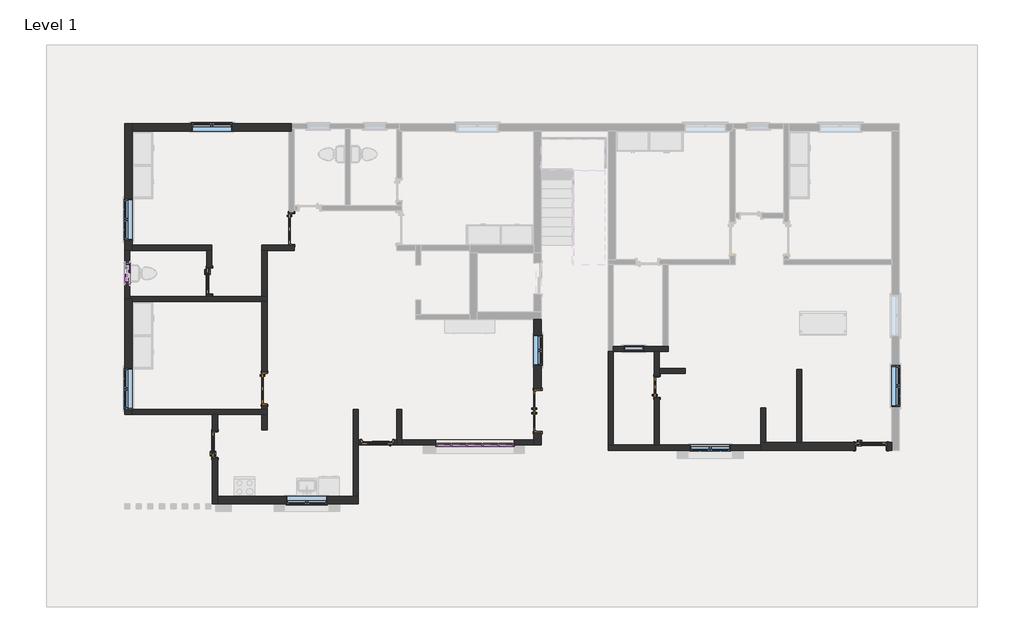
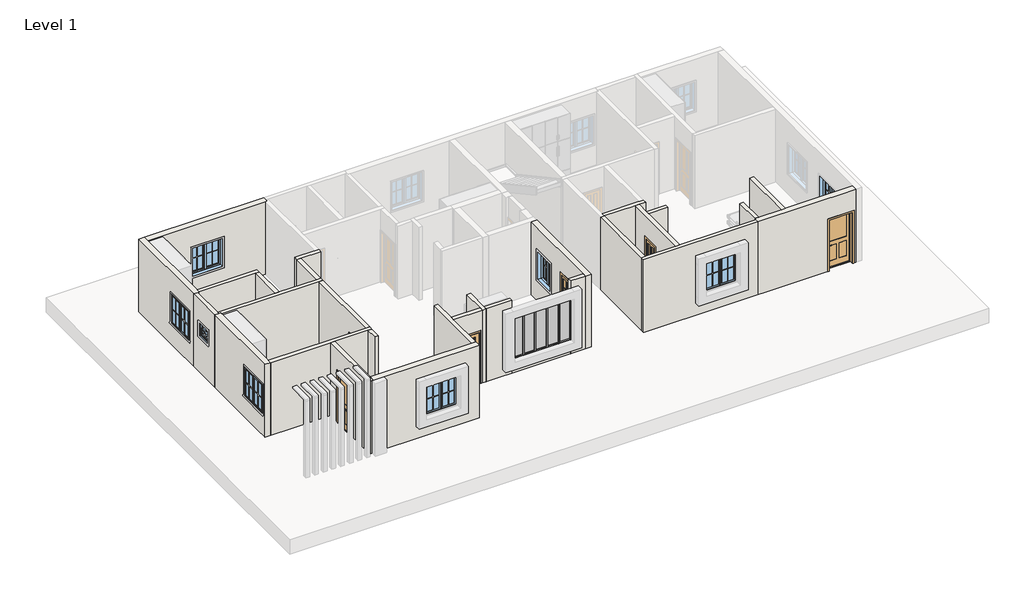
# One storey, part 1 of 3: 29 walls, 16 members, 9 windows, 8 doors, 5 plates.
"""IFC4 building model written with IfcOpenShell, lengths in millimetres."""

from ifc_helpers import new_model, si_unit, frame, origin, origin_with_axes, place, context, project, spatial, polyline, outline, extrude, faceted_brep, transform, mapped, element, save
from components import door_c9530512, door_0459eae1, door_3_x_7_64fb43ed, door_exterior_single_two_lite_3_x_7_37050820, door_interior_double_full_glass_wood_md_4_x_7_6b6f14de, door_interior_single_4_panel_wood_2_x_7_099afc9e, door_interior_single_4_panel_wood_bed_door_3_x_7_5a83478c, member_f5dffbef, member_20da7b42, member_5c57b440, member_8587bb6c, member_65702978, member_b71d7755, system_panel_glazed_d030299f, system_panel_glazed_4b6a6dc2, system_panel_glazed_d31e9b5d, system_panel_glazed_e2ad0beb, window_casement_double_3_x_4_2abbe05e, window_casement_double_4_x_4_9200f5ac, window_casement_double_4_x_4_83c2abfa, window_double_hung_2_x_2_0206a36d

model = new_model("IFC4")

# Units and contexts
model_context = context("Model", 3, world=origin())
ifc_project = project(units=[si_unit("LENGTHUNIT", "METRE", prefix="MILLI")], contexts=[model_context])

# Site, building, storey
site = spatial("IfcSite", under=ifc_project)
building = spatial("IfcBuilding", under=site)
storey = spatial("IfcBuildingStorey", under=building, Name="Level 1", Elevation=0.0)

# Doors
placement = place(None, origin())
door_shape = door_c9530512(model_context)
element("IfcDoor", 1, ObjectType="2'6\" X 7'", at=placement, inside=storey, context=model_context, shape_type="MappedRepresentation", body=[
    mapped(door_shape, transform((-9422.3392415, -3706.312639, 0.0), x_axis=(0.0, -1.0, 0.0), y_axis=(1.0, 0.0, 0.0), z_axis=(0.0, 0.0, 1.0))),
])
door_2_shape = door_0459eae1(model_context)
element("IfcDoor", 2, ObjectType="2'6\" X 7'", at=placement, inside=storey, context=model_context, shape_type="MappedRepresentation", body=[
    mapped(door_2_shape, transform((-9588.7286806, 1157.6726898, 0.0), x_axis=(0.0, 1.0, 0.0), y_axis=(-1.0, 0.0, 0.0), z_axis=(0.0, 0.0, 1.0))),
])
door_3_x_7_shape = door_3_x_7_64fb43ed(model_context)
element("IfcDoor", 3, ObjectType="3' X 7'", at=placement, inside=storey, context=model_context, shape_type="MappedRepresentation", body=[
    mapped(door_3_x_7_shape, transform((10074.0463194, -3754.0523102, 0.0), x_axis=(-1.0, 0.0, 0.0), y_axis=(0.0, -1.0, 0.0), z_axis=(0.0, 0.0, 1.0))),
])
door_exterior_single_two_lite_3_x_7_shape = door_exterior_single_two_lite_3_x_7_37050820(model_context)
element("IfcDoor", 4, ObjectType="Door-Exterior-Single-Two_Lite : 3' x 7'", at=placement, inside=storey, context=model_context, shape_type="MappedRepresentation", body=[
    mapped(door_exterior_single_two_lite_3_x_7_shape, transform((-4594.4536806, -3636.5773102, 0.0), x_axis=(-1.0, 0.0, 0.0), y_axis=(0.0, -1.0, 0.0), z_axis=(0.0, 0.0, 1.0))),
])
door_interior_double_full_glass_wood_md_4_x_7_shape = door_interior_double_full_glass_wood_md_4_x_7_6b6f14de(model_context)
element("IfcDoor", 5, ObjectType="Door-Interior-Double-Full Glass-Wood : MD 4' X 7'", at=placement, inside=storey, context=model_context, shape_type="MappedRepresentation", body=[
    mapped(door_interior_double_full_glass_wood_md_4_x_7_shape, transform((164.8713194, -2703.1273102, 0.0), x_axis=(0.0, 1.0, 0.0), y_axis=(-1.0, 0.0, 0.0), z_axis=(0.0, 0.0, 1.0))),
])
door_interior_single_4_panel_wood_2_x_7_shape = door_interior_single_4_panel_wood_2_x_7_099afc9e(model_context)
element("IfcDoor", 6, ObjectType="Door-Interior-Single-4_Panel-Wood : 2' X 7'", at=placement, inside=storey, context=model_context, shape_type="MappedRepresentation", body=[
    mapped(door_interior_single_4_panel_wood_2_x_7_shape, transform((3708.1713194, -1991.9273102, 0.0), x_axis=(0.0, 1.0, 0.0), y_axis=(-1.0, 0.0, 0.0), z_axis=(0.0, 0.0, 1.0))),
])
door_interior_single_4_panel_wood_bed_door_3_x_7_shape = door_interior_single_4_panel_wood_bed_door_3_x_7_5a83478c(model_context)
element("IfcDoor", 7, ObjectType="Door-Interior-Single-4_Panel-Wood : BED DOOR 3' X 7'", at=placement, inside=storey, context=model_context, shape_type="MappedRepresentation", body=[
    mapped(door_interior_single_4_panel_wood_bed_door_3_x_7_shape, transform((-7150.3286806, 2700.7226898, 0.0), x_axis=(0.0, -1.0, 0.0), y_axis=(1.0, 0.0, 0.0), z_axis=(0.0, 0.0, 1.0))),
])
element("IfcDoor", 8, ObjectType="Door-Interior-Single-4_Panel-Wood : BED DOOR 3' X 7'", at=placement, inside=storey, context=model_context, shape_type="MappedRepresentation", body=[
    mapped(door_interior_single_4_panel_wood_bed_door_3_x_7_shape, transform((-7950.4286806, -2042.7273102, 0.0), x_axis=(0.0, -1.0, 0.0), y_axis=(1.0, 0.0, 0.0), z_axis=(0.0, 0.0, 1.0))),
])

# Members
member_shape = member_f5dffbef(model_context)
element("IfcMember", 9, ObjectType="Rectangular Mullion : 1.5\" x 2.5\" rectangular", at=placement, inside=storey, context=model_context, shape_type="MappedRepresentation", body=[
    mapped(member_shape, transform((-568.5536806, -3719.1273102, 2438.4), x_axis=(0.0, 0.0, 1.0), y_axis=(0.0, -1.0, 0.0), z_axis=(1.0, 0.0, 0.0))),
])
member_2_shape = member_20da7b42(model_context)
element("IfcMember", 10, ObjectType="Rectangular Mullion : 1.5\" x 2.5\" rectangular", at=placement, inside=storey, context=model_context, shape_type="MappedRepresentation", body=[
    mapped(member_2_shape, transform((-2816.4536806, -3719.1273102, 609.6), x_axis=(0.0, 0.0, -1.0), y_axis=(0.0, -1.0, 0.0), z_axis=(-1.0, 0.0, 0.0))),
])
member_3_shape = member_5c57b440(model_context)
element("IfcMember", 11, ObjectType="Rectangular Mullion : 1.5\" x 2.5\" rectangular", at=placement, inside=storey, context=model_context, shape_type="MappedRepresentation", body=[
    mapped(member_3_shape, transform((-2397.3536806, -3719.1273102, 609.6), x_axis=(1.0, 0.0, 0.0), y_axis=(0.0, -1.0, 0.0), z_axis=(0.0, 0.0, -1.0))),
])
element("IfcMember", 12, ObjectType="Rectangular Mullion : 1.5\" x 2.5\" rectangular", at=placement, inside=storey, context=model_context, shape_type="MappedRepresentation", body=[
    mapped(member_3_shape, transform((-1940.1536806, -3719.1273102, 609.6), x_axis=(1.0, 0.0, 0.0), y_axis=(0.0, -1.0, 0.0), z_axis=(0.0, 0.0, -1.0))),
])
element("IfcMember", 13, ObjectType="Rectangular Mullion : 1.5\" x 2.5\" rectangular", at=placement, inside=storey, context=model_context, shape_type="MappedRepresentation", body=[
    mapped(member_3_shape, transform((-1470.2536806, -3719.1273102, 609.6), x_axis=(1.0, 0.0, 0.0), y_axis=(0.0, -1.0, 0.0), z_axis=(0.0, 0.0, -1.0))),
])
element("IfcMember", 14, ObjectType="Rectangular Mullion : 1.5\" x 2.5\" rectangular", at=placement, inside=storey, context=model_context, shape_type="MappedRepresentation", body=[
    mapped(member_3_shape, transform((-1000.3536806, -3719.1273102, 609.6), x_axis=(1.0, 0.0, 0.0), y_axis=(0.0, -1.0, 0.0), z_axis=(0.0, 0.0, -1.0))),
])
member_4_shape = member_8587bb6c(model_context)
element("IfcMember", 15, ObjectType="Rectangular Mullion : 1.5\" x 2.5\" rectangular", at=placement, inside=storey, context=model_context, shape_type="MappedRepresentation", body=[
    mapped(member_4_shape, transform((-2378.3036806, -3719.1273102, 609.6), x_axis=(0.0, 0.0, -1.0), y_axis=(0.0, -1.0, 0.0), z_axis=(-1.0, 0.0, 0.0))),
])
member_5_shape = member_65702978(model_context)
element("IfcMember", 16, ObjectType="Rectangular Mullion : 1.5\" x 2.5\" rectangular", at=placement, inside=storey, context=model_context, shape_type="MappedRepresentation", body=[
    mapped(member_5_shape, transform((-1921.1036806, -3719.1273102, 609.6), x_axis=(0.0, 0.0, -1.0), y_axis=(0.0, -1.0, 0.0), z_axis=(-1.0, 0.0, 0.0))),
])
element("IfcMember", 17, ObjectType="Rectangular Mullion : 1.5\" x 2.5\" rectangular", at=placement, inside=storey, context=model_context, shape_type="MappedRepresentation", body=[
    mapped(member_5_shape, transform((-1451.2036806, -3719.1273102, 609.6), x_axis=(0.0, 0.0, -1.0), y_axis=(0.0, -1.0, 0.0), z_axis=(-1.0, 0.0, 0.0))),
])
element("IfcMember", 18, ObjectType="Rectangular Mullion : 1.5\" x 2.5\" rectangular", at=placement, inside=storey, context=model_context, shape_type="MappedRepresentation", body=[
    mapped(member_shape, transform((-981.3036806, -3719.1273102, 609.6), x_axis=(0.0, 0.0, -1.0), y_axis=(0.0, -1.0, 0.0), z_axis=(-1.0, 0.0, 0.0))),
])
element("IfcMember", 19, ObjectType="Rectangular Mullion : 1.5\" x 2.5\" rectangular", at=placement, inside=storey, context=model_context, shape_type="MappedRepresentation", body=[
    mapped(member_2_shape, transform((-2416.4036806, -3719.1273102, 2438.4), x_axis=(0.0, 0.0, 1.0), y_axis=(0.0, -1.0, 0.0), z_axis=(1.0, 0.0, 0.0))),
])
element("IfcMember", 20, ObjectType="Rectangular Mullion : 1.5\" x 2.5\" rectangular", at=placement, inside=storey, context=model_context, shape_type="MappedRepresentation", body=[
    mapped(member_4_shape, transform((-1959.2036806, -3719.1273102, 2438.4), x_axis=(0.0, 0.0, 1.0), y_axis=(0.0, -1.0, 0.0), z_axis=(1.0, 0.0, 0.0))),
])
element("IfcMember", 21, ObjectType="Rectangular Mullion : 1.5\" x 2.5\" rectangular", at=placement, inside=storey, context=model_context, shape_type="MappedRepresentation", body=[
    mapped(member_5_shape, transform((-1489.3036806, -3719.1273102, 2438.4), x_axis=(0.0, 0.0, 1.0), y_axis=(0.0, -1.0, 0.0), z_axis=(1.0, 0.0, 0.0))),
])
element("IfcMember", 22, ObjectType="Rectangular Mullion : 1.5\" x 2.5\" rectangular", at=placement, inside=storey, context=model_context, shape_type="MappedRepresentation", body=[
    mapped(member_5_shape, transform((-1019.4036806, -3719.1273102, 2438.4), x_axis=(0.0, 0.0, 1.0), y_axis=(0.0, -1.0, 0.0), z_axis=(1.0, 0.0, 0.0))),
])
member_6_shape = member_b71d7755(model_context)
element("IfcMember", 23, ObjectType="Rectangular Mullion : 1.5\" x 2.5\" rectangular", at=placement, inside=storey, context=model_context, shape_type="MappedRepresentation", body=[
    mapped(member_6_shape, transform((-2854.5536806, -3719.1273102, 2438.4), x_axis=(-1.0, 0.0, 0.0), y_axis=(0.0, -1.0, 0.0), z_axis=(0.0, 0.0, 1.0))),
])
element("IfcMember", 24, ObjectType="Rectangular Mullion : 1.5\" x 2.5\" rectangular", at=placement, inside=storey, context=model_context, shape_type="MappedRepresentation", body=[
    mapped(member_6_shape, transform((-530.4536806, -3719.1273102, 609.6), x_axis=(1.0, 0.0, 0.0), y_axis=(0.0, -1.0, 0.0), z_axis=(0.0, 0.0, -1.0))),
])

# Plates
system_panel_glazed_shape = system_panel_glazed_d030299f(model_context)
element("IfcPlate", 25, ObjectType="System Panel : Glazed", at=placement, inside=storey, context=model_context, shape_type="MappedRepresentation", body=[
    mapped(system_panel_glazed_shape, transform((-2616.4286806, -3719.1273102, 647.7), x_axis=(1.0, 0.0, 0.0), y_axis=(0.0, 1.0, 0.0), z_axis=(0.0, 0.0, 1.0))),
])
system_panel_glazed_2_shape = system_panel_glazed_4b6a6dc2(model_context)
element("IfcPlate", 26, ObjectType="System Panel : Glazed", at=placement, inside=storey, context=model_context, shape_type="MappedRepresentation", body=[
    mapped(system_panel_glazed_2_shape, transform((-2168.7536806, -3719.1273102, 647.7), x_axis=(1.0, 0.0, 0.0), y_axis=(0.0, 1.0, 0.0), z_axis=(0.0, 0.0, 1.0))),
])
system_panel_glazed_3_shape = system_panel_glazed_d31e9b5d(model_context)
element("IfcPlate", 27, ObjectType="System Panel : Glazed", at=placement, inside=storey, context=model_context, shape_type="MappedRepresentation", body=[
    mapped(system_panel_glazed_3_shape, transform((-1705.2036806, -3719.1273102, 647.7), x_axis=(1.0, 0.0, 0.0), y_axis=(0.0, 1.0, 0.0), z_axis=(0.0, 0.0, 1.0))),
])
element("IfcPlate", 28, ObjectType="System Panel : Glazed", at=placement, inside=storey, context=model_context, shape_type="MappedRepresentation", body=[
    mapped(system_panel_glazed_3_shape, transform((-1235.3036806, -3719.1273102, 647.7), x_axis=(1.0, 0.0, 0.0), y_axis=(0.0, 1.0, 0.0), z_axis=(0.0, 0.0, 1.0))),
])
system_panel_glazed_4_shape = system_panel_glazed_e2ad0beb(model_context)
element("IfcPlate", 29, ObjectType="System Panel : Glazed", at=placement, inside=storey, context=model_context, shape_type="MappedRepresentation", body=[
    mapped(system_panel_glazed_4_shape, transform((-774.9286806, -3719.1273102, 647.7), x_axis=(1.0, 0.0, 0.0), y_axis=(0.0, 1.0, 0.0), z_axis=(0.0, 0.0, 1.0))),
])

# Walls
element("IfcWall", 30, ObjectType="6\"", at=placement, inside=storey, context=model_context, shape_type="Brep", body=[
    faceted_brep([(-11871.5536806, 2072.0726898, 0.0), (-9661.7536806, 2072.0726898, 0.0), (-9509.3536806, 2072.0726898, 0.0), (-9509.3536806, 2072.0726898, 3048.0), (-9661.7536806, 2072.0726898, 3048.0), (-11871.5536806, 2072.0726898, 3048.0), (-11871.5536806, 2224.4726898, 0.0), (-11871.5536806, 2224.4726898, 3048.0), (-9509.3536806, 2224.4726898, 3048.0), (-9509.3536806, 2224.4726898, 0.0)], [[[0, 1, 2, 3, 4, 5]], [[6, 7, 8, 9]], [[2, 1, 0, 6, 9]], [[5, 4, 3, 8, 7]], [[0, 5, 7, 6]], [[3, 2, 9, 8]]]),
])
element("IfcWall", 31, ObjectType="6\"", at=placement, inside=storey, context=model_context, shape_type="Brep", body=[
    faceted_brep([(-8023.4774184, 2072.0726898, 0.0), (-7871.0774184, 2072.0726898, 0.0), (-7070.9536806, 2072.0726898, 0.0), (-7070.9536806, 2072.0726898, 3048.0), (-7871.0774184, 2072.0726898, 3048.0), (-8023.4774184, 2072.0726898, 3048.0), (-8023.4774184, 2224.4726898, 3048.0), (-7223.3536806, 2224.4726898, 3048.0), (-7070.9536806, 2224.4726898, 3048.0), (-7070.9536806, 2224.4726898, 2159.0), (-7223.3536806, 2224.4726898, 2159.0), (-7223.3536806, 2224.4726898, 0.0), (-8023.4774184, 2224.4726898, 0.0), (-7223.3536806, 2218.1226898, 0.0), (-7070.9536806, 2218.1226898, 0.0), (-7070.9536806, 2218.1226898, 2159.0), (-7223.3536806, 2218.1226898, 2159.0)], [[[0, 1, 2, 3, 4, 5]], [[6, 7, 8, 9, 10, 11, 12]], [[2, 1, 0, 12, 11, 13, 14]], [[5, 4, 3, 8, 7, 6]], [[3, 2, 14, 15, 9, 8]], [[0, 5, 6, 12]], [[16, 13, 11, 10]], [[13, 16, 15, 14]], [[15, 16, 10, 9]]]),
])
element("IfcWall", 32, ObjectType="6\"", at=placement, inside=storey, context=model_context, shape_type="Brep", body=[
    faceted_brep([(53.7463194, -3566.7273102, 0.0), (-530.4536806, -3566.7273102, 0.0), (-530.4536806, -3566.7273102, 609.6), (-530.4536806, -3566.7273102, 2438.4), (-530.4536806, -3566.7273102, 3048.0), (53.7463194, -3566.7273102, 3048.0), (53.7463194, -3719.1273102, 0.0), (53.7463194, -3719.1273102, 3048.0), (-530.4536806, -3719.1273102, 3048.0), (-530.4536806, -3719.1273102, 2438.4), (-530.4536806, -3719.1273102, 609.6), (-530.4536806, -3719.1273102, 0.0)], [[[0, 1, 2, 3, 4, 5]], [[6, 7, 8, 9, 10, 11]], [[1, 0, 6, 11]], [[5, 4, 8, 7]], [[0, 5, 7, 6]], [[1, 11, 10, 9, 8, 4, 3, 2]]]),
])
element("IfcWall", 33, ObjectType="6\"", at=placement, inside=storey, context=model_context, shape_type="Brep", body=[
    faceted_brep([(-3870.5536806, -3719.1273102, 0.0), (-3870.5536806, -3566.7273102, 0.0), (-3870.5536806, -2652.3273102, 0.0), (-3870.5536806, -2652.3273102, 3048.0), (-3870.5536806, -3566.7273102, 3048.0), (-3870.5536806, -3719.1273102, 3048.0), (-4022.9536806, -3719.1273102, 0.0), (-4022.9536806, -3719.1273102, 3048.0), (-4022.9536806, -3566.7273102, 3048.0), (-4022.9536806, -2652.3273102, 3048.0), (-4022.9536806, -2652.3273102, 0.0), (-4022.9536806, -3566.7273102, 0.0)], [[[0, 1, 2, 3, 4, 5]], [[6, 7, 8, 9, 10, 11]], [[2, 1, 0, 6, 11, 10]], [[3, 2, 10, 9]], [[5, 4, 3, 9, 8, 7]], [[0, 5, 7, 6]]]),
])
element("IfcWall", 34, ObjectType="6\"", at=placement, inside=storey, context=model_context, shape_type="SweptSolid", body=[
    extrude(outline(polyline([(700.4726898, 3048.0), (2072.0726898, 3048.0), (2072.0726898, 0.0), (1564.0726898, 0.0), (1564.0726898, 2159.0), (751.2726898, 2159.0), (751.2726898, 0.0), (700.4726898, 0.0), (700.4726898, 3048.0)])), frame((-9661.7536806, 0.0, 0.0), z_axis=(1.0, 0.0, 0.0), x_axis=(0.0, 1.0, 0.0)), (0.0, 0.0, 1.0), 152.4),
])
element("IfcWall", 35, ObjectType="6\"", at=placement, inside=storey, context=model_context, shape_type="SweptSolid", body=[
    extrude(outline(polyline([(-7871.0774184, 2072.0726898), (-7871.0774184, 700.4726898), (-8023.4774184, 700.4726898), (-8023.4774184, 2072.0726898), (-7871.0774184, 2072.0726898)])), origin_with_axes(), (0.0, 0.0, 1.0), 3048.0),
])
element("IfcWall", 36, ObjectType="6\"", at=placement, inside=storey, context=model_context, shape_type="Brep", body=[
    faceted_brep([(-12100.1536806, 2072.0726898, 0.0), (-12100.1536806, 624.2726898, 0.0), (-12100.1536806, 624.2726898, 3048.0), (-12100.1536806, 2072.0726898, 3048.0), (-12100.1536806, 1691.0726898, 2120.9), (-12100.1536806, 1081.4726898, 2120.9), (-12100.1536806, 1081.4726898, 1524.0), (-12100.1536806, 1691.0726898, 1524.0), (-11947.7536806, 2072.0726898, 0.0), (-11947.7536806, 2072.0726898, 3048.0), (-11947.7536806, 700.4726898, 3048.0), (-11947.7536806, 624.2726898, 3048.0), (-11947.7536806, 624.2726898, 0.0), (-11947.7536806, 700.4726898, 0.0), (-11947.7536806, 1691.0726898, 2120.9), (-11947.7536806, 1691.0726898, 1524.0), (-11947.7536806, 1081.4726898, 1524.0), (-11947.7536806, 1081.4726898, 2120.9)], [[[0, 1, 2, 3], [4, 5, 6, 7]], [[8, 9, 10, 11, 12, 13], [14, 15, 16, 17]], [[1, 0, 8, 13, 12]], [[2, 1, 12, 11]], [[3, 2, 11, 10, 9]], [[0, 3, 9, 8]], [[15, 14, 4, 7]], [[16, 15, 7, 6]], [[17, 16, 6, 5]], [[14, 17, 5, 4]]]),
])
element("IfcWall", 37, ObjectType="6\"", at=placement, inside=storey, context=model_context, shape_type="Brep", body=[
    faceted_brep([(-11871.5536806, 548.0726898, 0.0), (-8023.4536806, 548.0726898, 0.0), (-7871.0536806, 548.0726898, 0.0), (-7871.0536806, 548.0726898, 3048.0), (-8023.4536806, 548.0726898, 3048.0), (-11871.5536806, 548.0726898, 3048.0), (-11947.7536806, 700.4726898, 0.0), (-11947.7536806, 700.4726898, 3048.0), (-9661.7536806, 700.4726898, 3048.0), (-9509.3536806, 700.4726898, 3048.0), (-8023.4774184, 700.4726898, 3048.0), (-7871.0536806, 700.4726898, 3048.0), (-7871.0536806, 700.4726898, 0.0), (-8023.4774184, 700.4726898, 0.0), (-9509.3536806, 700.4726898, 0.0), (-9661.7536806, 700.4726898, 0.0), (-11871.5536806, 624.2726898, 0.0), (-11947.7536806, 624.2726898, 0.0), (-11947.7536806, 624.2726898, 3048.0), (-11871.5536806, 624.2726898, 3048.0)], [[[0, 1, 2, 3, 4, 5]], [[6, 7, 8, 9, 10, 11, 12, 13, 14, 15]], [[2, 1, 0, 16, 17, 6, 15, 14, 13, 12]], [[5, 4, 3, 11, 10, 9, 8, 7, 18, 19]], [[0, 5, 19, 16]], [[19, 18, 17, 16]], [[18, 7, 6, 17]], [[3, 2, 12, 11]]]),
])
element("IfcWall", 38, ObjectType="6\"", at=placement, inside=storey, context=model_context, shape_type="Brep", body=[
    faceted_brep([(-11871.5536806, -2804.7273102, 0.0), (-9495.3642415, -2804.7273102, 0.0), (-9342.9642415, -2804.7273102, 0.0), (-8023.4536806, -2804.7273102, 0.0), (-7871.0536806, -2804.7273102, 0.0), (-7871.0536806, -2804.7273102, 3048.0), (-8023.4536806, -2804.7273102, 3048.0), (-9342.9642415, -2804.7273102, 3048.0), (-9495.3642415, -2804.7273102, 3048.0), (-11871.5536806, -2804.7273102, 3048.0), (-11871.5536806, -2652.3273102, 0.0), (-11871.5536806, -2652.3273102, 914.4), (-11871.5536806, -2652.3273102, 2133.6), (-11871.5536806, -2652.3273102, 3048.0), (-8023.4536806, -2652.3273102, 3048.0), (-7871.0536806, -2652.3273102, 3048.0), (-7871.0536806, -2652.3273102, 0.0), (-8023.4536806, -2652.3273102, 0.0)], [[[0, 1, 2, 3, 4, 5, 6, 7, 8, 9]], [[10, 11, 12, 13, 14, 15, 16, 17]], [[4, 3, 2, 1, 0, 10, 17, 16]], [[9, 8, 7, 6, 5, 15, 14, 13]], [[5, 4, 16, 15]], [[0, 9, 13, 12, 11, 10]]]),
])
element("IfcWall", 39, ObjectType="6\"", at=placement, inside=storey, context=model_context, shape_type="SweptSolid", body=[
    extrude(outline(polyline([(-2652.3273102, 3048.0), (548.0726898, 3048.0), (548.0726898, 0.0), (-1560.1273102, 0.0), (-1560.1273102, 2159.0), (-2525.3273102, 2159.0), (-2525.3273102, 0.0), (-2652.3273102, 0.0), (-2652.3273102, 3048.0)])), frame((-8023.4536806, 0.0, 0.0), z_axis=(1.0, 0.0, 0.0), x_axis=(0.0, 1.0, 0.0)), (0.0, 0.0, 1.0), 152.4),
])
element("IfcWall", 40, ObjectType="6\"", at=placement, inside=storey, context=model_context, shape_type="Brep", body=[
    faceted_brep([(-9342.9642415, -2804.7273102, 3048.0), (-9342.9642415, -5243.1273102, 3048.0), (-9342.9642415, -5471.7273102, 3048.0), (-9342.9642415, -5471.7273102, 0.0), (-9342.9642415, -5243.1273102, 0.0), (-9342.9642415, -4112.712639, 0.0), (-9342.9642415, -4112.712639, 2159.0), (-9342.9642415, -3299.912639, 2159.0), (-9342.9642415, -3299.912639, 0.0), (-9342.9642415, -2804.7273102, 0.0), (-9495.3642415, -5471.7273102, 3048.0), (-9495.3642415, -2804.7273102, 3048.0), (-9495.3642415, -2804.7273102, 0.0), (-9495.3642415, -3299.912639, 0.0), (-9495.3642415, -3299.912639, 2159.0), (-9495.3642415, -4112.712639, 2159.0), (-9495.3642415, -4112.712639, 0.0), (-9495.3642415, -5471.7273102, 0.0)], [[[0, 1, 2, 3, 4, 5, 6, 7, 8, 9]], [[10, 11, 12, 13, 14, 15, 16, 17]], [[3, 17, 16, 5, 4]], [[12, 9, 8, 13]], [[2, 1, 0, 11, 10]], [[15, 6, 5, 16]], [[6, 15, 14, 7]], [[7, 14, 13, 8]], [[3, 2, 10, 17]], [[0, 9, 12, 11]]]),
])
element("IfcWall", 41, ObjectType="6\"", at=placement, inside=storey, context=model_context, shape_type="Brep", body=[
    faceted_brep([(-5165.9536806, -5243.1273102, 0.0), (-5165.9536806, -3719.1273102, 0.0), (-5165.9536806, -3566.7273102, 0.0), (-5165.9536806, -2652.3273102, 0.0), (-5165.9536806, -2652.3273102, 3048.0), (-5165.9536806, -3566.7273102, 3048.0), (-5165.9536806, -3719.1273102, 3048.0), (-5165.9536806, -5243.1273102, 3048.0), (-5318.3536806, -5243.1273102, 0.0), (-5318.3536806, -5243.1273102, 3048.0), (-5318.3536806, -2652.3273102, 3048.0), (-5318.3536806, -2652.3273102, 0.0)], [[[0, 1, 2, 3, 4, 5, 6, 7]], [[8, 9, 10, 11]], [[3, 2, 1, 0, 8, 11]], [[4, 3, 11, 10]], [[7, 6, 5, 4, 10, 9]], [[0, 7, 9, 8]]]),
])
element("IfcWall", 42, ObjectType="6\"", at=placement, inside=storey, context=model_context, shape_type="SweptSolid", body=[
    extrude(outline(polyline([(-8023.4536806, -3261.9273102), (-8023.4536806, -2804.7273102), (-7871.0536806, -2804.7273102), (-7871.0536806, -3261.9273102), (-8023.4536806, -3261.9273102)])), origin_with_axes(), (0.0, 0.0, 1.0), 3048.0),
])
element("IfcWall", 43, ObjectType="6\"", at=placement, inside=storey, context=model_context, shape_type="Brep", body=[
    faceted_brep([(2415.9463194, -937.8273102, 0.0), (3635.1463194, -937.8273102, 0.0), (3787.5463194, -937.8273102, 0.0), (4041.5463194, -937.8273102, 0.0), (4041.5463194, -937.8273102, 3048.0), (3787.5463194, -937.8273102, 3048.0), (3635.1463194, -937.8273102, 3048.0), (2415.9463194, -937.8273102, 3048.0), (2720.7463194, -937.8273102, 1511.3), (3330.3463194, -937.8273102, 1511.3), (3330.3463194, -937.8273102, 914.4), (2720.7463194, -937.8273102, 914.4), (2415.9463194, -785.4273102, 0.0), (2415.9463194, -785.4273102, 3048.0), (3889.1463194, -785.4273102, 3048.0), (4041.5463194, -785.4273102, 3048.0), (4041.5463194, -785.4273102, 0.0), (3889.1463194, -785.4273102, 0.0), (2720.7463194, -785.4273102, 1511.3), (2720.7463194, -785.4273102, 914.4), (3330.3463194, -785.4273102, 914.4), (3330.3463194, -785.4273102, 1511.3)], [[[0, 1, 2, 3, 4, 5, 6, 7], [8, 9, 10, 11]], [[12, 13, 14, 15, 16, 17], [18, 19, 20, 21]], [[3, 2, 1, 0, 12, 17, 16]], [[7, 6, 5, 4, 15, 14, 13]], [[0, 7, 13, 12]], [[4, 3, 16, 15]], [[19, 18, 8, 11]], [[20, 19, 11, 10]], [[21, 20, 10, 9]], [[18, 21, 9, 8]]]),
])
element("IfcWall", 44, ObjectType="6\"", at=placement, inside=storey, context=model_context, shape_type="SweptSolid", body=[
    extrude(outline(polyline([(8016.6463194, -1471.2273102), (8016.6463194, -3642.9273102), (7864.2463194, -3642.9273102), (7864.2463194, -1471.2273102), (8016.6463194, -1471.2273102)])), origin_with_axes(), (0.0, 0.0, 1.0), 3048.0),
])
element("IfcWall", 45, ObjectType="6\"", at=placement, inside=storey, context=model_context, shape_type="SweptSolid", body=[
    extrude(outline(polyline([(6949.8463194, -2614.2273102), (6949.8463194, -3642.9273102), (6797.4463194, -3642.9273102), (6797.4463194, -2614.2273102), (6949.8463194, -2614.2273102)])), origin_with_axes(), (0.0, 0.0, 1.0), 3048.0),
])
element("IfcWall", 46, ObjectType="6\"", at=placement, inside=storey, context=model_context, shape_type="Brep", body=[
    faceted_brep([(6797.4463194, -3719.1273102, 0.0), (3787.5463194, -3719.1273102, 0.0), (3635.1463194, -3719.1273102, 0.0), (2415.9463194, -3719.1273102, 0.0), (2263.5463194, -3719.1273102, 0.0), (2263.5463194, -3719.1273102, 3048.0), (2415.9463194, -3719.1273102, 3048.0), (3635.1463194, -3719.1273102, 3048.0), (3787.5463194, -3719.1273102, 3048.0), (6797.4463194, -3719.1273102, 3048.0), (4682.8963194, -3719.1273102, 2133.6), (4682.8963194, -3719.1273102, 914.4), (5902.0963194, -3719.1273102, 914.4), (5902.0963194, -3719.1273102, 2133.6), (6797.4463194, -3871.5273102, 0.0), (6797.4463194, -3871.5273102, 3048.0), (2263.5463194, -3871.5273102, 3048.0), (2263.5463194, -3871.5273102, 0.0), (4682.8963194, -3871.5273102, 2133.6), (5902.0963194, -3871.5273102, 2133.6), (5902.0963194, -3871.5273102, 914.4), (4682.8963194, -3871.5273102, 914.4)], [[[0, 1, 2, 3, 4, 5, 6, 7, 8, 9], [10, 11, 12, 13]], [[14, 15, 16, 17], [18, 19, 20, 21]], [[4, 3, 2, 1, 0, 14, 17]], [[9, 8, 7, 6, 5, 16, 15]], [[0, 9, 15, 14]], [[5, 4, 17, 16]], [[11, 10, 18, 21]], [[12, 11, 21, 20]], [[13, 12, 20, 19]], [[10, 13, 19, 18]]]),
])
element("IfcWall", 47, ObjectType="6\"", at=placement, inside=storey, context=model_context, shape_type="Brep", body=[
    faceted_brep([(3787.5463194, -937.8273102, 3048.0), (3787.5463194, -1433.1273102, 3048.0), (3787.5463194, -1585.5273102, 3048.0), (3787.5463194, -3719.1273102, 3048.0), (3787.5463194, -3719.1273102, 0.0), (3787.5463194, -2322.1273102, 0.0), (3787.5463194, -2322.1273102, 2159.0), (3787.5463194, -1661.7273102, 2159.0), (3787.5463194, -1661.7273102, 0.0), (3787.5463194, -1585.5273102, 0.0), (3787.5463194, -1433.1273102, 0.0), (3787.5463194, -937.8273102, 0.0), (3635.1463194, -3719.1273102, 3048.0), (3635.1463194, -937.8273102, 3048.0), (3635.1463194, -937.8273102, 0.0), (3635.1463194, -1661.7273102, 0.0), (3635.1463194, -1661.7273102, 2159.0), (3635.1463194, -2322.1273102, 2159.0), (3635.1463194, -2322.1273102, 0.0), (3635.1463194, -3719.1273102, 0.0)], [[[0, 1, 2, 3, 4, 5, 6, 7, 8, 9, 10, 11]], [[12, 13, 14, 15, 16, 17, 18, 19]], [[4, 19, 18, 5]], [[14, 11, 10, 9, 8, 15]], [[3, 2, 1, 0, 13, 12]], [[4, 3, 12, 19]], [[0, 11, 14, 13]], [[7, 16, 15, 8]], [[16, 7, 6, 17]], [[17, 6, 5, 18]]]),
])
element("IfcWall", 48, ObjectType="6\"", at=placement, inside=storey, context=model_context, shape_type="SweptSolid", body=[
    extrude(outline(polyline([(2415.9463194, -937.8273102), (2415.9463194, -3719.1273102), (2263.5463194, -3719.1273102), (2263.5463194, -937.8273102), (2415.9463194, -937.8273102)])), origin_with_axes(), (0.0, 0.0, 1.0), 3048.0),
])
element("IfcWall", 49, ObjectType="6\"", at=placement, inside=storey, context=model_context, shape_type="SweptSolid", body=[
    extrude(outline(polyline([(4549.5463194, -1585.5273102), (3787.5463194, -1585.5273102), (3787.5463194, -1433.1273102), (4549.5463194, -1433.1273102), (4549.5463194, -1585.5273102)])), origin_with_axes(), (0.0, 0.0, 1.0), 3048.0),
])
element("IfcWall", 50, ObjectType="6\"", at=placement, inside=storey, context=model_context, shape_type="SweptSolid", body=[
    extrude(outline(polyline([(3048.0, -4022.9536806), (3048.0, -5165.9536806), (0.0, -5165.9536806), (0.0, -5102.4536806), (2235.2, -5102.4536806), (2235.2, -4086.4536806), (0.0, -4086.4536806), (0.0, -4022.9536806), (3048.0, -4022.9536806)])), frame((0.0, -3719.1273102, 0.0), z_axis=(0.0, 1.0, 0.0), x_axis=(0.0, 0.0, 1.0)), (0.0, 0.0, 1.0), 152.4),
])
element("IfcWall", 51, ObjectType="6\"", at=placement, inside=storey, context=model_context, shape_type="Brep", body=[
    faceted_brep([(-2854.5536806, -3566.7273102, 3048.0), (-2854.5536806, -3566.7273102, 2438.4), (-2854.5536806, -3566.7273102, 609.6), (-2854.5536806, -3566.7273102, 0.0), (-3870.5536806, -3566.7273102, 0.0), (-3870.5536806, -3566.7273102, 3048.0), (-2854.5536806, -3719.1273102, 0.0), (-2854.5536806, -3719.1273102, 609.6), (-2854.5536806, -3719.1273102, 2438.4), (-2854.5536806, -3719.1273102, 3048.0), (-3870.5536806, -3719.1273102, 3048.0), (-3870.5536806, -3719.1273102, 0.0)], [[[0, 1, 2, 3, 4, 5]], [[6, 7, 8, 9, 10, 11]], [[4, 3, 6, 11]], [[0, 5, 10, 9]], [[5, 4, 11, 10]], [[0, 9, 8, 7, 6, 3, 2, 1]]]),
])
element("IfcWall", 52, ObjectType="6\"", at=placement, inside=storey, context=model_context, shape_type="SweptSolid", body=[
    extrude(outline(polyline([(-530.4536806, -3719.1273102), (-2854.5536806, -3719.1273102), (-2854.5536806, -3566.7273102), (-530.4536806, -3566.7273102), (-530.4536806, -3719.1273102)])), origin_with_axes(), (0.0, 0.0, 1.0), 609.6),
])
element("IfcWall", 53, ObjectType="9\"", at=placement, inside=storey, context=model_context, shape_type="Brep", body=[
    faceted_brep([(-11871.5536806, 5615.3726898, 0.0), (-7223.3536806, 5615.3726898, 0.0), (-7147.1536806, 5615.3726898, 0.0), (-7147.1536806, 5615.3726898, 3048.0), (-7223.3536806, 5615.3726898, 3048.0), (-11871.5536806, 5615.3726898, 3048.0), (-8899.7536806, 5615.3726898, 2133.6), (-8899.7536806, 5615.3726898, 914.4), (-10118.9536806, 5615.3726898, 914.4), (-10118.9536806, 5615.3726898, 2133.6), (-11871.5536806, 5843.9726898, 0.0), (-11871.5536806, 5843.9726898, 3048.0), (-7147.1536806, 5843.9726898, 3048.0), (-7147.1536806, 5843.9726898, 0.0), (-8899.7536806, 5843.9726898, 2133.6), (-10118.9536806, 5843.9726898, 2133.6), (-10118.9536806, 5843.9726898, 914.4), (-8899.7536806, 5843.9726898, 914.4), (-7147.1536806, 5691.5726898, 0.0), (-7147.1536806, 5691.5726898, 3048.0)], [[[0, 1, 2, 3, 4, 5], [6, 7, 8, 9]], [[10, 11, 12, 13], [14, 15, 16, 17]], [[2, 1, 0, 10, 13, 18]], [[3, 2, 18, 13, 12, 19]], [[5, 4, 3, 19, 12, 11]], [[0, 5, 11, 10]], [[7, 6, 14, 17]], [[8, 7, 17, 16]], [[9, 8, 16, 15]], [[6, 9, 15, 14]]]),
])
element("IfcWall", 54, ObjectType="9\"", at=placement, inside=storey, context=model_context, shape_type="Brep", body=[
    faceted_brep([(53.7463194, -3719.1273102, 3048.0), (53.7463194, -3566.7273102, 3048.0), (53.7463194, 14.6726898, 3048.0), (53.7463194, 14.6726898, 0.0), (53.7463194, -2068.1273102, 0.0), (53.7463194, -2068.1273102, 2159.0), (53.7463194, -3338.1273102, 2159.0), (53.7463194, -3338.1273102, 0.0), (53.7463194, -3566.7273102, 0.0), (53.7463194, -3719.1273102, 0.0), (53.7463194, -1356.9273102, 2133.6), (53.7463194, -1356.9273102, 914.4), (53.7463194, -442.5273102, 914.4), (53.7463194, -442.5273102, 2133.6), (282.3463194, 14.6726898, 3048.0), (282.3463194, -3719.1273102, 3048.0), (282.3463194, -3719.1273102, 0.0), (282.3463194, -3338.1273102, 0.0), (282.3463194, -3338.1273102, 2159.0), (282.3463194, -2068.1273102, 2159.0), (282.3463194, -2068.1273102, 0.0), (282.3463194, 14.6726898, 0.0), (282.3463194, -1356.9273102, 2133.6), (282.3463194, -442.5273102, 2133.6), (282.3463194, -442.5273102, 914.4), (282.3463194, -1356.9273102, 914.4)], [[[0, 1, 2, 3, 4, 5, 6, 7, 8, 9], [10, 11, 12, 13]], [[14, 15, 16, 17, 18, 19, 20, 21], [22, 23, 24, 25]], [[3, 21, 20, 4]], [[16, 9, 8, 7, 17]], [[2, 1, 0, 15, 14]], [[3, 2, 14, 21]], [[0, 9, 16, 15]], [[19, 5, 4, 20]], [[5, 19, 18, 6]], [[6, 18, 17, 7]], [[11, 10, 22, 25]], [[12, 11, 25, 24]], [[13, 12, 24, 23]], [[10, 13, 23, 22]]]),
])
element("IfcWall", 55, ObjectType="9\"", at=placement, inside=storey, context=model_context, shape_type="Brep", body=[
    faceted_brep([(-11871.5536806, 2072.0726898, 0.0), (-11871.5536806, 2224.4726898, 0.0), (-11871.5536806, 5615.3726898, 0.0), (-11871.5536806, 5843.9726898, 0.0), (-11871.5536806, 5843.9726898, 3048.0), (-11871.5536806, 5615.3726898, 3048.0), (-11871.5536806, 2224.4726898, 3048.0), (-11871.5536806, 2072.0726898, 3048.0), (-11871.5536806, 3596.0726898, 2133.6), (-11871.5536806, 3596.0726898, 914.4), (-11871.5536806, 2376.8726898, 914.4), (-11871.5536806, 2376.8726898, 2133.6), (-12100.1536806, 2072.0726898, 0.0), (-12100.1536806, 2072.0726898, 3048.0), (-12100.1536806, 5843.9726898, 3048.0), (-12100.1536806, 5843.9726898, 0.0), (-12100.1536806, 3596.0726898, 2133.6), (-12100.1536806, 2376.8726898, 2133.6), (-12100.1536806, 2376.8726898, 914.4), (-12100.1536806, 3596.0726898, 914.4), (-11947.7536806, 2072.0726898, 0.0), (-11947.7536806, 2072.0726898, 3048.0)], [[[0, 1, 2, 3, 4, 5, 6, 7], [8, 9, 10, 11]], [[12, 13, 14, 15], [16, 17, 18, 19]], [[3, 2, 1, 0, 20, 12, 15]], [[7, 6, 5, 4, 14, 13, 21]], [[4, 3, 15, 14]], [[0, 7, 21, 13, 12, 20]], [[9, 8, 16, 19]], [[10, 9, 19, 18]], [[11, 10, 18, 17]], [[8, 11, 17, 16]]]),
])
element("IfcWall", 56, ObjectType="9\"", at=placement, inside=storey, context=model_context, shape_type="Brep", body=[
    faceted_brep([(-11871.5536806, -2804.7273102, 0.0), (-11871.5536806, -2652.3273102, 0.0), (-11871.5536806, 548.0726898, 0.0), (-11871.5536806, 624.2726898, 0.0), (-11871.5536806, 624.2726898, 3048.0), (-11871.5536806, 548.0726898, 3048.0), (-11871.5536806, -2652.3273102, 3048.0), (-11871.5536806, -2804.7273102, 3048.0), (-11871.5536806, -1433.1273102, 2133.6), (-11871.5536806, -1433.1273102, 914.4), (-11871.5536806, -2652.3273102, 914.4), (-11871.5536806, -2652.3273102, 2133.6), (-12100.1536806, -2804.7273102, 0.0), (-12100.1536806, -2804.7273102, 3048.0), (-12100.1536806, 624.2726898, 3048.0), (-12100.1536806, 624.2726898, 0.0), (-12100.1536806, -1433.1273102, 2133.6), (-12100.1536806, -2652.3273102, 2133.6), (-12100.1536806, -2652.3273102, 914.4), (-12100.1536806, -1433.1273102, 914.4), (-11947.7536806, 624.2726898, 0.0), (-11947.7536806, 624.2726898, 3048.0)], [[[0, 1, 2, 3, 4, 5, 6, 7], [8, 9, 10, 11]], [[12, 13, 14, 15], [16, 17, 18, 19]], [[3, 2, 1, 0, 12, 15, 20]], [[4, 3, 20, 15, 14, 21]], [[7, 6, 5, 4, 21, 14, 13]], [[0, 7, 13, 12]], [[9, 8, 16, 19]], [[10, 9, 19, 18]], [[11, 10, 18, 17]], [[8, 11, 17, 16]]]),
])
element("IfcWall", 57, ObjectType="9\"", at=placement, inside=storey, context=model_context, shape_type="Brep", body=[
    faceted_brep([(6797.4463194, -3642.9273102, 3048.0), (6949.8463194, -3642.9273102, 3048.0), (7864.2463194, -3642.9273102, 3048.0), (8016.6463194, -3642.9273102, 3048.0), (10683.6463194, -3642.9273102, 3048.0), (10683.6463194, -3642.9273102, 0.0), (10556.6463194, -3642.9273102, 0.0), (10556.6463194, -3642.9273102, 2159.0), (9591.4463194, -3642.9273102, 2159.0), (9591.4463194, -3642.9273102, 0.0), (8016.6463194, -3642.9273102, 0.0), (7864.2463194, -3642.9273102, 0.0), (6949.8463194, -3642.9273102, 0.0), (6797.4463194, -3642.9273102, 0.0), (10683.6463194, -3871.5273102, 3048.0), (6797.4463194, -3871.5273102, 3048.0), (6797.4463194, -3871.5273102, 0.0), (9591.4463194, -3871.5273102, 0.0), (9591.4463194, -3871.5273102, 2159.0), (10556.6463194, -3871.5273102, 2159.0), (10556.6463194, -3871.5273102, 0.0), (10683.6463194, -3871.5273102, 0.0), (6797.4463194, -3719.1273102, 0.0), (6797.4463194, -3719.1273102, 3048.0)], [[[0, 1, 2, 3, 4, 5, 6, 7, 8, 9, 10, 11, 12, 13]], [[14, 15, 16, 17, 18, 19, 20, 21]], [[5, 21, 20, 6]], [[16, 22, 13, 12, 11, 10, 9, 17]], [[4, 3, 2, 1, 0, 23, 15, 14]], [[5, 4, 14, 21]], [[0, 13, 22, 16, 15, 23]], [[8, 18, 17, 9]], [[18, 8, 7, 19]], [[19, 7, 6, 20]]]),
])
element("IfcWall", 58, ObjectType="9\"", at=placement, inside=storey, context=model_context, shape_type="Brep", body=[
    faceted_brep([(-5165.9536806, -5243.1273102, 0.0), (-5318.3536806, -5243.1273102, 0.0), (-9342.9642415, -5243.1273102, 0.0), (-9342.9642415, -5243.1273102, 3048.0), (-5318.3536806, -5243.1273102, 3048.0), (-5165.9536806, -5243.1273102, 3048.0), (-7299.5536806, -5243.1273102, 2133.6), (-7299.5536806, -5243.1273102, 914.4), (-6080.3536806, -5243.1273102, 914.4), (-6080.3536806, -5243.1273102, 2133.6), (-5165.9536806, -5471.7273102, 0.0), (-5165.9536806, -5471.7273102, 3048.0), (-9342.9642415, -5471.7273102, 3048.0), (-9342.9642415, -5471.7273102, 0.0), (-7299.5536806, -5471.7273102, 2133.6), (-6080.3536806, -5471.7273102, 2133.6), (-6080.3536806, -5471.7273102, 914.4), (-7299.5536806, -5471.7273102, 914.4)], [[[0, 1, 2, 3, 4, 5], [6, 7, 8, 9]], [[10, 11, 12, 13], [14, 15, 16, 17]], [[2, 1, 0, 10, 13]], [[5, 4, 3, 12, 11]], [[0, 5, 11, 10]], [[3, 2, 13, 12]], [[7, 6, 14, 17]], [[8, 7, 17, 16]], [[9, 8, 16, 15]], [[6, 9, 15, 14]]]),
])

# Windows
window_casement_double_3_x_4_shape = window_casement_double_3_x_4_2abbe05e(model_context)
element("IfcWindow", 59, ObjectType="Window-Casement-Double : 3' X 4'", at=placement, inside=storey, context=model_context, shape_type="MappedRepresentation", body=[
    mapped(window_casement_double_3_x_4_shape, transform((168.0463194, -899.7273102, 0.0), x_axis=(0.0, -1.0, 0.0), y_axis=(1.0, 0.0, 0.0), z_axis=(0.0, 0.0, 1.0))),
])
window_casement_double_4_x_4_shape = window_casement_double_4_x_4_9200f5ac(model_context)
element("IfcWindow", 60, ObjectType="Window-Casement-Double : 4' X 4'", at=placement, inside=storey, context=model_context, shape_type="MappedRepresentation", body=[
    mapped(window_casement_double_4_x_4_shape, transform((-9509.3536806, 5729.6726898, 0.0), x_axis=(1.0, 0.0, 0.0), y_axis=(0.0, 1.0, 0.0), z_axis=(0.0, 0.0, 1.0))),
])
element("IfcWindow", 61, ObjectType="Window-Casement-Double : 4' X 4'", at=placement, inside=storey, context=model_context, shape_type="MappedRepresentation", body=[
    mapped(window_casement_double_4_x_4_shape, transform((10797.9463194, -1966.5273102, 0.0), x_axis=(0.0, -1.0, 0.0), y_axis=(1.0, 0.0, 0.0), z_axis=(0.0, 0.0, 1.0))),
])
element("IfcWindow", 62, ObjectType="Window-Casement-Double : 4' X 4'", at=placement, inside=storey, context=model_context, shape_type="MappedRepresentation", body=[
    mapped(window_casement_double_4_x_4_shape, transform((-11985.8536806, -2042.7273102, 0.0), x_axis=(0.0, 1.0, 0.0), y_axis=(-1.0, 0.0, 0.0), z_axis=(0.0, 0.0, 1.0))),
])
element("IfcWindow", 63, ObjectType="Window-Casement-Double : 4' X 4'", at=placement, inside=storey, context=model_context, shape_type="MappedRepresentation", body=[
    mapped(window_casement_double_4_x_4_shape, transform((-11985.8536806, 2986.4726898, 0.0), x_axis=(0.0, 1.0, 0.0), y_axis=(-1.0, 0.0, 0.0), z_axis=(0.0, 0.0, 1.0))),
])
element("IfcWindow", 64, ObjectType="Window-Casement-Double : 4' X 4'", at=placement, inside=storey, context=model_context, shape_type="MappedRepresentation", body=[
    mapped(window_casement_double_4_x_4_shape, transform((-6689.9536806, -5357.4273102, 0.0), x_axis=(-1.0, 0.0, 0.0), y_axis=(0.0, -1.0, 0.0), z_axis=(0.0, 0.0, 1.0))),
])
window_casement_double_4_x_4_2_shape = window_casement_double_4_x_4_83c2abfa(model_context)
element("IfcWindow", 65, ObjectType="Window-Casement-Double : 4' X 4'", at=placement, inside=storey, context=model_context, shape_type="MappedRepresentation", body=[
    mapped(window_casement_double_4_x_4_2_shape, transform((5292.4963194, -3795.3273102, 0.0), x_axis=(-1.0, 0.0, 0.0), y_axis=(0.0, -1.0, 0.0), z_axis=(0.0, 0.0, 1.0))),
])
window_double_hung_2_x_2_shape = window_double_hung_2_x_2_0206a36d(model_context)
element("IfcWindow", 66, ObjectType="Window-Double-Hung : 2' X 2'", at=placement, inside=storey, context=model_context, shape_type="MappedRepresentation", body=[
    mapped(window_double_hung_2_x_2_shape, transform((-12023.9536806, 1386.2726898, 609.6), x_axis=(0.0, -1.0, 0.0), y_axis=(1.0, 0.0, 0.0), z_axis=(0.0, 0.0, 1.0))),
])
element("IfcWindow", 67, ObjectType="Window-Double-Hung : 2' X 2'", at=placement, inside=storey, context=model_context, shape_type="MappedRepresentation", body=[
    mapped(window_double_hung_2_x_2_shape, transform((3025.5463194, -861.6273102, 0.0), x_axis=(1.0, 0.0, 0.0), y_axis=(0.0, 1.0, 0.0), z_axis=(0.0, 0.0, 1.0))),
])

save(model, "model.ifc")

# Revit data of these elements
# Type "2'6\" X 7'"
#   Type Mark = "15"
#   Assembly Code = "B2030100"
#   Analytic Construction = "French door, wood frame with single glass"
#   Top Rail = 0' - 4 3/4"
#   Threshold Offset [instance default] = 0' - 0 1/2"
#   Thickness = 0' - 1 3/8"
#   Thermal Resistance (R) = 1.0696 (h·ft²·°F)/BTU
#   Swing Angle [instance default] = 90.00°
#   Stiles = 0' - 4 3/4"
#   Rough Width = 2' - 8"
#   Rough Height = 7' - 1"
#   Lock Rail = 0' - 7 1/8"
#   Height = 7' - 0"
#   Width = 2' - 6"
#   Heat Transfer Coefficient (U) = 0.9350 BTU/(h·ft²·°F)
#   Door Offset [instance default] = 0' - 0"
#   Bottom Rail = 0' - 9 1/2"
#   Threshold [instance default] = yes
#   Function = 1
#   Exterior Trim [instance default] = yes
#   Trim Material = Cherry
#   Threshold Material = Cherry
#   Panel Material = Cherry
#   Glazing = Glass
#   Frame Material = Cherry
#   Door Handle Material = Aluminum
#   Visual Light Transmittance = 0
#   Solar Heat Gain Coefficient = 0
#   Wall Closure = (empty or 0)
#   Construction Type = (empty or 0)
# Type "3' X 7'"
#   Type Mark = "16"
#   Assembly Code = "B2030100"
#   Analytic Construction = "French door, wood frame with single glass"
#   Top Rail = 0' - 4 3/4"
#   Threshold Offset [instance default] = 0' - 0 1/2"
#   Thickness = 0' - 1 3/8"
#   Thermal Resistance (R) = 1.0696 (h·ft²·°F)/BTU
#   Swing Angle [instance default] = 90.00°
#   Stiles = 0' - 4 3/4"
#   Rough Width = 3' - 2"
#   Rough Height = 7' - 1"
#   Lock Rail = 0' - 7 1/8"
#   Height = 7' - 0"
#   Width = 3' - 0"
#   Heat Transfer Coefficient (U) = 0.9350 BTU/(h·ft²·°F)
#   Door Offset [instance default] = 0' - 0"
#   Bottom Rail = 0' - 9 1/2"
#   Threshold [instance default] = yes
#   Function = 1
#   Exterior Trim [instance default] = yes
#   Trim Material = Cherry
#   Threshold Material = Cherry
#   Panel Material = Cherry
#   Glazing = Glass
#   Frame Material = Cherry
#   Door Handle Material = Aluminum
#   Visual Light Transmittance = 0
#   Solar Heat Gain Coefficient = 0
#   Wall Closure = (empty or 0)
#   Construction Type = (empty or 0)
# Type "Door-Exterior-Single-Two_Lite : 3' x 7'"
#   Type Mark = "19"
#   Assembly Code = "B2030100"
#   Analytic Construction = "Metal frame, double glass door"
#   Top Rail = 0' - 6"
#   Threshold Offset [instance default] = 0' - 0 1/2"
#   Threshold Length [instance default] = 3' - 4"
#   Thickness = 0' - 1 3/4"
#   Thermal Resistance (R) = 1.3794 (h·ft²·°F)/BTU
#   Swing Angle [instance default] = 90.00°
#   Strike Height = 3' - 4"
#   Stiles = 0' - 6"
#   Rough Width [instance default] = 3' - 4"
#   Rough Height [instance default] = 7' - 4"
#   MFOpeningHeight [instance default] = 0' - 4"
#   MFOpeningWidth [instance default] = 0' - 4"
#   Lock Rail = 0' - 7 1/2"
#   Heat Transfer Coefficient (U) = 0.7250 BTU/(h·ft²·°F)
#   Glass Thickness = 0' - 0 3/4"
#   Inset Calculate [instance default] = 0' - 4"
#   Masonry Inset [instance default] = 0' - 1"
#   Height = 7' - 0"
#   Width = 3' - 0"
#   Masonry Frame Depth = 0' - 5 3/4"
#   Bottom Rail = 0' - 10"
#   Masonry Frame [instance default] = yes
#   Function = 1
#   Threshold [instance default] = yes
#   Dry Wall Frame [instance default] = no
#   Threshold Material = none
#   Panic Bar Material = Metal - Stainless Steel
#   Panel Material = Metal - Painted - Grey
#   Glass Stop Material = Metal - Painted - Grey
#   Exterior Pull Material = Metal - Stainless Steel
#   Frame Material = Metal - Painted - Grey
#   Visual Light Transmittance = 0
#   Solar Heat Gain Coefficient = 0
#   Wall Closure = (empty or 0)
# Type "Door-Interior-Double-Full Glass-Wood : MD 4' X 7'"
#   Type Mark = "9"
#   Assembly Code = "C1020300"
#   Analytic Construction = "French door, wood frame with single glass"
#   Top Rail = 0' - 4 11/16"
#   Thickness = 0' - 1 3/8"
#   Thermal Resistance (R) = 1.0696 (h·ft²·°F)/BTU
#   Swing Angle [instance default] = 90.00°
#   Stiles = 0' - 4 3/4"
#   Rough Width = 4' - 2"
#   Rough Height = 7' - 1"
#   Panel Width = 2' - 0"
#   Height = 7' - 0"
#   Width = 4' - 0"
#   Heat Transfer Coefficient (U) = 0.9350 BTU/(h·ft²·°F)
#   Bottom Rail = 0' - 9 1/8"
#   Show Grill [instance default] = yes
#   Trim Material = Cherry
#   Panel Material = Cherry
#   Frame Material = Cherry
#   Door Handle Material = Aluminum
#   Visual Light Transmittance = 0
#   Solar Heat Gain Coefficient = 0
#   Wall Closure = (empty or 0)
#   Function = (empty or 0)
# Type "Door-Interior-Single-4_Panel-Wood : 2' X 7'"
#   Type Mark = "17"
#   Assembly Code = "C1020300"
#   Analytic Construction = "Wooden"
#   Top Rail = 0' - 4 11/16"
#   Thickness = 0' - 1 3/8"
#   Thermal Resistance (R) = 2.5876 (h·ft²·°F)/BTU
#   Swing Angle [instance default] = 90.00°
#   Stiles = 0' - 4 3/4"
#   Rough Width = 2' - 2"
#   Rough Height = 7' - 1"
#   Mullion = 0' - 4 1/2"
#   Lock Rail = 0' - 7 1/2"
#   Height = 7' - 0"
#   Width = 2' - 0"
#   Heat Transfer Coefficient (U) = 0.3865 BTU/(h·ft²·°F)
#   Bottom Rail = 0' - 9 1/8"
#   Trim Material = Cherry
#   Panel Material = Cherry
#   Frame Material = Cherry
#   Door Handle Material = Aluminum
#   Visual Light Transmittance = 0
#   Solar Heat Gain Coefficient = 0
#   Wall Closure = (empty or 0)
#   Function = (empty or 0)
# Type "Door-Interior-Single-4_Panel-Wood : BED DOOR 3' X 7'"
#   Type Mark = "13"
#   Assembly Code = "C1020300"
#   Analytic Construction = "Wooden"
#   Top Rail = 0' - 4 11/16"
#   Thickness = 0' - 1 3/8"
#   Thermal Resistance (R) = 2.5876 (h·ft²·°F)/BTU
#   Swing Angle [instance default] = 90.00°
#   Stiles = 0' - 4 3/4"
#   Rough Width = 3' - 2"
#   Rough Height = 7' - 1"
#   Mullion = 0' - 4 1/2"
#   Lock Rail = 0' - 7 1/2"
#   Height = 7' - 0"
#   Width = 3' - 0"
#   Heat Transfer Coefficient (U) = 0.3865 BTU/(h·ft²·°F)
#   Bottom Rail = 0' - 9 1/8"
#   Trim Material = Cherry
#   Panel Material = Cherry
#   Frame Material = Cherry
#   Door Handle Material = Aluminum
#   Visual Light Transmittance = 0
#   Solar Heat Gain Coefficient = 0
#   Wall Closure = (empty or 0)
#   Function = (empty or 0)
# Type "Rectangular Mullion : 1.5\" x 2.5\" rectangular"
#   built-in parameter 1007304 = 0.208333 (stored number, unit not read)
#   built-in parameter 1007301 = 0.0625 (stored number, unit not read)
#   built-in parameter 1007300 = 0.0625 (stored number, unit not read)
# Type "System Panel : Glazed"
#   Construction Type Id = "GSP4R"
#   Analytic Construction = "1/8 in Pilkington single glazing"
#   Visual Light Transmittance = 0.9
#   Solar Heat Gain Coefficient = 0.86
#   Heat Transfer Coefficient (U) = 1.18115 BTU/(h·ft²·°F)
#   Define Thermal Properties by = 1
# Type "6\""
#   Assembly Code = "B2010"
#   Layers, outside or top first: 0' - 6" "wall" (function 1)
# Type "9\""
#   Assembly Code = "B2010"
#   Layers, outside or top first: 0' - 9" "wall" (function 1)
# Type "Window-Casement-Double : 3' X 4'"
#   Type Mark = "20"
#   Fire Rating = "0.5h"
#   Assembly Code = "B2020100"
#   Analytic Construction = "Double glazing - domestic"
#   Frame Extension [instance default] = 0' - 0 1/4"
#   Window Inset [instance default] = 0' - 0"
#   Wall Thickness [instance default] = 0' - 6"
#   Interior Wall Closure [instance default] = 0' - 2 1/4"
#   Half Width = 1' - 6"
#   Visual Light Transmittance = 0.81
#   Thermal Resistance (R) = 1.8146 (h·ft²·°F)/BTU
#   Solar Heat Gain Coefficient = 0.76
#   Rough Width = 3' - 0 1/2"
#   Rough Height = 4' - 0 1/2"
#   Height = 4' - 0"
#   Heat Transfer Coefficient (U) = 0.5511 BTU/(h·ft²·°F)
#   Exterior Wall Closure [instance default] = 0' - 1 1/4"
#   Extension Jamb [instance default] = 0' - 2 1/4"
#   Default Sill Height = 3' - 0"
#   Width = 3' - 0"
#   Muntin Visibility = yes
#   Interior Trim Visibility [instance default] = yes
#   Exterior Trim Visibility [instance default] = yes
#   Extension Jamb Visibility [instance default] = yes
#   Interior Trim Material = Wood - Stained
#   Muntin Pattern = Muntin Pattern_2x2 : Muntin Pattern_2x2
#   Interior Trim = Trim-Window-Interior-Flat : Picture Frame
#   Interior Frame Material = Wood - Stained
#   Glass Panel Material = Glass
#   Exterior Trim Material = Clad - White
#   Exterior Trim = Trim-Window-Exterior-Flat : with Sill
#   Exterior Frame Material = Clad - White
#   Wall Closure = (empty or 0)
# Type "Window-Casement-Double : 4' X 4'"
#   Type Mark = "19"
#   Fire Rating = "0.5h"
#   Assembly Code = "B2020100"
#   Analytic Construction = "Double glazing - domestic"
#   Frame Extension [instance default] = 0' - 0 1/4"
#   Window Inset [instance default] = 0' - 0"
#   Wall Thickness [instance default] = 0' - 6"
#   Interior Wall Closure [instance default] = 0' - 2 1/4"
#   Half Width = 2' - 0"
#   Visual Light Transmittance = 0.81
#   Thermal Resistance (R) = 1.8146 (h·ft²·°F)/BTU
#   Solar Heat Gain Coefficient = 0.76
#   Rough Width = 4' - 0 1/2"
#   Rough Height = 4' - 0 1/2"
#   Height = 4' - 0"
#   Heat Transfer Coefficient (U) = 0.5511 BTU/(h·ft²·°F)
#   Exterior Wall Closure [instance default] = 0' - 1 1/4"
#   Extension Jamb [instance default] = 0' - 2 1/4"
#   Default Sill Height = 3' - 0"
#   Width = 4' - 0"
#   Muntin Visibility = yes
#   Interior Trim Visibility [instance default] = yes
#   Exterior Trim Visibility [instance default] = yes
#   Extension Jamb Visibility [instance default] = yes
#   Interior Trim Material = Wood - Stained
#   Muntin Pattern = Muntin Pattern_2x2 : Muntin Pattern_2x2
#   Interior Trim = Trim-Window-Interior-Flat : Picture Frame
#   Interior Frame Material = Wood - Stained
#   Glass Panel Material = Glass
#   Exterior Trim Material = Clad - White
#   Exterior Trim = Trim-Window-Exterior-Flat : with Sill
#   Exterior Frame Material = Clad - White
#   Wall Closure = (empty or 0)
# Type "Window-Double-Hung : 2' X 2'"
#   Type Mark = "25"
#   Fire Rating = "0.5h"
#   Construction Type Id = "DG-DR"
#   Assembly Code = "B2020100"
#   Analytic Construction = "Double glazing - domestic"
#   Wall Thickness [instance default] = 0' - 6"
#   Window Inset [instance default] = 0' - 0"
#   Visual Light Transmittance = 0.81
#   Thermal Resistance (R) = 1.8146 (h·ft²·°F)/BTU
#   Solar Heat Gain Coefficient = 0.76
#   Muntin Width = 1' - 6"
#   Muntin Height = 0' - 7 7/8"
#   Interior Wall Closure [instance default] = 0' - 1 1/2"
#   Rough Width = 2' - 0 1/2"
#   Rough Height = 2' - 0"
#   Frame Extension [instance default] = 0' - 1 1/4"
#   Exterior Wall Closure [instance default] = 0' - 0 1/2"
#   Extension Jamb [instance default] = 0' - 1 1/2"
#   Heat Transfer Coefficient (U) = 0.5511 BTU/(h·ft²·°F)
#   Height = 1' - 11 1/2"
#   Width = 2' - 0"
#   Top Muntin Visibility = yes
#   Indicator Visibility [instance default] = yes
#   Extension Jamb Visibility [instance default] = yes
#   Interior Trim Visibility [instance default] = yes
#   Exterior Trim Visibility [instance default] = yes
#   Define Thermal Properties by = 1
#   Bottom Muntin Visibility = yes
#   Muntin Pattern = Muntin Pattern_2x2 : Muntin Pattern_2x2
#   Interior Trim Material = Wood - Stained
#   Interior Trim = Trim-Window-Interior-Flat : Picture Frame
#   Exterior Trim Material = Clad - White
#   Exterior Trim = Trim-Window-Exterior-Flat : with Sill
#   Glass Panel Material = Glass
#   Exterior Frame Material = Clad - White
#   Interior Frame Material = Wood - Stained
#   Wall Closure = (empty or 0)
# Elements 1, 2 (IfcDoor, "2'6\" X 7'")
#   Threshold Offset = 0' - 0 1/2"
#   Swing Angle = 90.00°
#   Door Offset = 0' - 0"
#   Threshold = yes
#   Exterior Trim = yes
#   Phase Created = New Construction
#   Materials on its faces: "Cherry", "Aluminum", "Glass"
# Element 3 (IfcDoor, "3' X 7'")
#   Threshold Offset = 0' - 0 1/2"
#   Swing Angle = 90.00°
#   Door Offset = 0' - 0"
#   Threshold = yes
#   Exterior Trim = yes
#   Phase Created = New Construction
#   Materials on its faces: "Cherry", "Aluminum", "Glass"
# Element 4 (IfcDoor, "Door-Exterior-Single-Two_Lite : 3' x 7'")
#   Threshold Offset = 0' - 0 1/2"
#   Threshold Length = 3' - 4"
#   Swing Angle = 90.00°
#   Rough Width = 3' - 4"
#   Rough Height = 7' - 4"
#   Masonry Inset = 0' - 1"
#   MFOpeningWidth = 0' - 4"
#   MFOpeningHeight = 0' - 4"
#   Inset Calculate = 0' - 4"
#   Threshold = yes
#   Masonry Frame = yes
#   Dry Wall Frame = no
#   Phase Created = New Construction
#   Materials on its faces: "Metal - Painted - Grey", "Metal - Stainless Steel", "Glass"
# Element 5 (IfcDoor, "Door-Interior-Double-Full Glass-Wood : MD 4' X 7'")
#   Swing Angle = 90.00°
#   Show Grill = yes
#   Phase Created = New Construction
#   Materials on its faces: "Cherry", "Aluminum", "Glass"
# Element 6 (IfcDoor, "Door-Interior-Single-4_Panel-Wood : 2' X 7'")
#   Swing Angle = 90.00°
#   Phase Created = New Construction
#   Materials on its faces: "Cherry", "Aluminum"
# Elements 7, 8 (IfcDoor, "Door-Interior-Single-4_Panel-Wood : BED DOOR 3' X 7'")
#   Swing Angle = 90.00°
#   Phase Created = New Construction
#   Materials on its faces: "Cherry", "Aluminum"
# Elements 9, 10, 11, 12, 13, 14, 15, 16, 17, 18, 19, 20, 21, 22, 23, 24 (IfcMember, "Rectangular Mullion : 1.5\" x 2.5\" rectangular")
#   Phase Created = New Construction
#   Materials on its faces: "Aluminum"
# Elements 25, 26, 27, 28, 29 (IfcPlate, "System Panel : Glazed")
#   Phase Created = New Construction
#   Materials on its faces: "Glass"
# Elements 30, 32, 33, 34, 35, 36, 37, 38, 39, 40, 41, 42, 43, 44, 45, 46, 47, 48, 49, 50, 51 (IfcWall, "6\"")
#   Top Offset = 0' - 0"
#   Base Offset = 0' - 0"
#   wall height = 10' - 0"
#   Phase Created = New Construction
#   Base Constraint = Level 1
#   Top Constraint = Level 2
#   Materials on its faces: "wall"
# Element 31 (IfcWall, "6\"")
#   Top Offset = 0' - 0"
#   Base Offset = 0' - 0"
#   wall height = 10' - 0"
#   Phase Created = New Construction
#   Base Constraint = Level 1
#   Top Constraint = Level 2
#   Materials on its faces: "wall", "exterior wall"
# Element 52 (IfcWall, "6\"")
#   Top Offset = 0' - 0"
#   Base Offset = 0' - 0"
#   Unconnected Height = 2' - 0"
#   wall height = 2' - 0"
#   Phase Created = New Construction
#   Base Constraint = Level 1
#   Materials on its faces: "wall"
# Elements 53, 54, 55, 56, 57, 58 (IfcWall, "9\"")
#   Top Offset = 0' - 0"
#   Base Offset = 0' - 0"
#   wall height = 10' - 0"
#   Phase Created = New Construction
#   Base Constraint = Level 1
